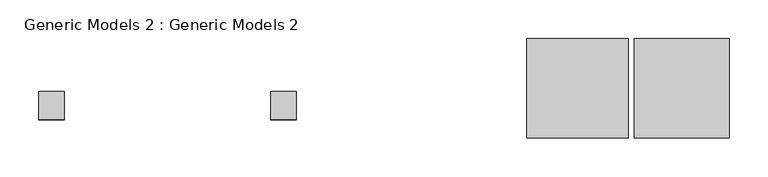
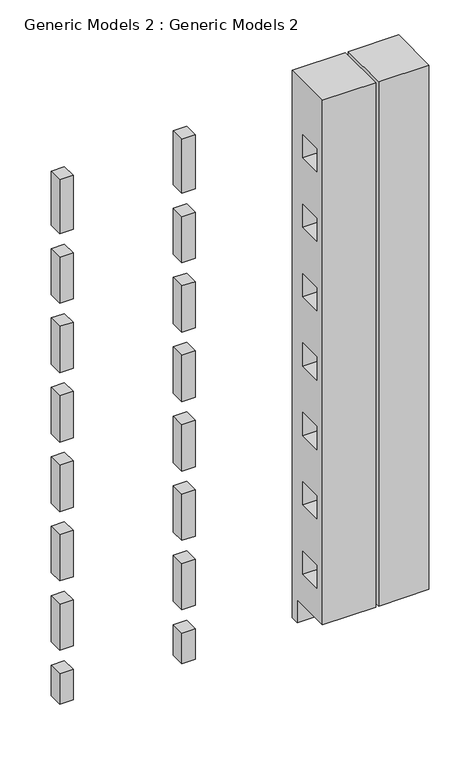
"""IFC4 building model written with IfcOpenShell, lengths in millimetres: proxy geometry, Generic Models 2 : Generic Models 2."""

from ifc_helpers import new_model, si_unit, frame, origin, place, context, project, spatial, polyline, outline, extrude, source, transform, mapped, element, save


def generic_models_2_generic_models_2_e4755291(model_context):
    return source(origin(), model_context, "Body", "SweptSolid", [
        extrude(outline(polyline([(-2976.5029848, -6160.9896754), (-2976.5029848, -6197.2837816), (-3009.36382, -6197.2837816), (-3009.36382, -6160.9896754), (-2976.5029848, -6160.9896754)])), frame((0.0, 0.0, 834.3679056), z_axis=(0.0, 0.0, 1.0), x_axis=(1.0, 0.0, 0.0)), (0.0, 0.0, 1.0), 140.0),
        extrude(outline(polyline([(-2676.5029848, -6160.9896754), (-2676.5029848, -6197.2837816), (-2709.36382, -6197.2837816), (-2709.36382, -6160.9896754), (-2676.5029848, -6160.9896754)])), frame((0.0, 0.0, 834.3679056), z_axis=(0.0, 0.0, 1.0), x_axis=(1.0, 0.0, 0.0)), (0.0, 0.0, 1.0), 140.0),
        extrude(outline(polyline([(-6092.2648653, 974.3679056), (-6092.2648653, -445.6320944), (-6113.8685722, -445.6320944), (-6113.8685722, -385.6320944), (-6220.9896754, -385.6320944), (-6220.9896754, 974.3679056), (-6092.2648653, 974.3679056)]), holes=[polyline([(-6137.2837816, 834.3679056), (-6197.2837816, 834.3679056), (-6197.2837816, 774.3679056), (-6137.2837816, 774.3679056), (-6137.2837816, 834.3679056)]), polyline([(-6137.2837816, 654.3679056), (-6197.2837816, 654.3679056), (-6197.2837816, 594.3679056), (-6137.2837816, 594.3679056), (-6137.2837816, 654.3679056)]), polyline([(-6137.2837816, 474.3679056), (-6197.2837816, 474.3679056), (-6197.2837816, 414.3679056), (-6137.2837816, 414.3679056), (-6137.2837816, 474.3679056)]), polyline([(-6137.2837816, 294.3679056), (-6197.2837816, 294.3679056), (-6197.2837816, 234.3679056), (-6137.2837816, 234.3679056), (-6137.2837816, 294.3679056)]), polyline([(-6137.2837816, 114.3679056), (-6197.2837816, 114.3679056), (-6197.2837816, 54.3679056), (-6137.2837816, 54.3679056), (-6137.2837816, 114.3679056)]), polyline([(-6137.2837816, -65.6320944), (-6197.2837816, -65.6320944), (-6197.2837816, -125.6320944), (-6137.2837816, -125.6320944), (-6137.2837816, -65.6320944)]), polyline([(-6137.2837816, -245.6320944), (-6197.2837816, -245.6320944), (-6197.2837816, -305.6320944), (-6137.2837816, -305.6320944), (-6137.2837816, -245.6320944)])]), frame((-2378.5868425, 0.0, 0.0), z_axis=(1.0, 0.0, 0.0), x_axis=(0.0, 1.0, 0.0)), (0.0, 0.0, 1.0), 130.7324377),
        extrude(outline(polyline([(-6092.2648653, 974.3679056), (-6092.2648653, -445.6320944), (-6113.8685722, -445.6320944), (-6113.8685722, -385.6320944), (-6220.9896754, -385.6320944), (-6220.9896754, 974.3679056), (-6092.2648653, 974.3679056)]), holes=[polyline([(-6137.2837816, 834.3679056), (-6197.2837816, 834.3679056), (-6197.2837816, 774.3679056), (-6137.2837816, 774.3679056), (-6137.2837816, 834.3679056)]), polyline([(-6137.2837816, 654.3679056), (-6197.2837816, 654.3679056), (-6197.2837816, 594.3679056), (-6137.2837816, 594.3679056), (-6137.2837816, 654.3679056)]), polyline([(-6137.2837816, 474.3679056), (-6197.2837816, 474.3679056), (-6197.2837816, 414.3679056), (-6137.2837816, 414.3679056), (-6137.2837816, 474.3679056)]), polyline([(-6137.2837816, 294.3679056), (-6197.2837816, 294.3679056), (-6197.2837816, 234.3679056), (-6137.2837816, 234.3679056), (-6137.2837816, 294.3679056)]), polyline([(-6137.2837816, 114.3679056), (-6197.2837816, 114.3679056), (-6197.2837816, 54.3679056), (-6137.2837816, 54.3679056), (-6137.2837816, 114.3679056)]), polyline([(-6137.2837816, -65.6320944), (-6197.2837816, -65.6320944), (-6197.2837816, -125.6320944), (-6137.2837816, -125.6320944), (-6137.2837816, -65.6320944)]), polyline([(-6137.2837816, -245.6320944), (-6197.2837816, -245.6320944), (-6197.2837816, -305.6320944), (-6137.2837816, -305.6320944), (-6137.2837816, -245.6320944)])]), frame((-2240.2544048, 0.0, 0.0), z_axis=(1.0, 0.0, 0.0), x_axis=(0.0, 1.0, 0.0)), (0.0, 0.0, 1.0), 123.0190663),
        extrude(outline(polyline([(-2976.5029848, -6160.9896754), (-2976.5029848, -6197.2837816), (-3009.36382, -6197.2837816), (-3009.36382, -6160.9896754), (-2976.5029848, -6160.9896754)])), frame((0.0, 0.0, 654.3679056), z_axis=(0.0, 0.0, 1.0), x_axis=(1.0, 0.0, 0.0)), (0.0, 0.0, 1.0), 120.0),
        extrude(outline(polyline([(-2676.5029848, -6160.9896754), (-2676.5029848, -6197.2837816), (-2709.36382, -6197.2837816), (-2709.36382, -6160.9896754), (-2676.5029848, -6160.9896754)])), frame((0.0, 0.0, 654.3679056), z_axis=(0.0, 0.0, 1.0), x_axis=(1.0, 0.0, 0.0)), (0.0, 0.0, 1.0), 120.0),
        extrude(outline(polyline([(-2976.5029848, -6160.9896754), (-2976.5029848, -6197.2837816), (-3009.36382, -6197.2837816), (-3009.36382, -6160.9896754), (-2976.5029848, -6160.9896754)])), frame((0.0, 0.0, 474.3679056), z_axis=(0.0, 0.0, 1.0), x_axis=(1.0, 0.0, 0.0)), (0.0, 0.0, 1.0), 120.0),
        extrude(outline(polyline([(-2676.5029848, -6160.9896754), (-2676.5029848, -6197.2837816), (-2709.36382, -6197.2837816), (-2709.36382, -6160.9896754), (-2676.5029848, -6160.9896754)])), frame((0.0, 0.0, 474.3679056), z_axis=(0.0, 0.0, 1.0), x_axis=(1.0, 0.0, 0.0)), (0.0, 0.0, 1.0), 120.0),
        extrude(outline(polyline([(-2976.5029848, -6160.9896754), (-2976.5029848, -6197.2837816), (-3009.36382, -6197.2837816), (-3009.36382, -6160.9896754), (-2976.5029848, -6160.9896754)])), frame((0.0, 0.0, 294.3679056), z_axis=(0.0, 0.0, 1.0), x_axis=(1.0, 0.0, 0.0)), (0.0, 0.0, 1.0), 120.0),
        extrude(outline(polyline([(-2676.5029848, -6160.9896754), (-2676.5029848, -6197.2837816), (-2709.36382, -6197.2837816), (-2709.36382, -6160.9896754), (-2676.5029848, -6160.9896754)])), frame((0.0, 0.0, 294.3679056), z_axis=(0.0, 0.0, 1.0), x_axis=(1.0, 0.0, 0.0)), (0.0, 0.0, 1.0), 120.0),
        extrude(outline(polyline([(-2976.5029848, -6160.9896754), (-2976.5029848, -6197.2837816), (-3009.36382, -6197.2837816), (-3009.36382, -6160.9896754), (-2976.5029848, -6160.9896754)])), frame((0.0, 0.0, 114.3679056), z_axis=(0.0, 0.0, 1.0), x_axis=(1.0, 0.0, 0.0)), (0.0, 0.0, 1.0), 120.0),
        extrude(outline(polyline([(-2676.5029848, -6160.9896754), (-2676.5029848, -6197.2837816), (-2709.36382, -6197.2837816), (-2709.36382, -6160.9896754), (-2676.5029848, -6160.9896754)])), frame((0.0, 0.0, 114.3679056), z_axis=(0.0, 0.0, 1.0), x_axis=(1.0, 0.0, 0.0)), (0.0, 0.0, 1.0), 120.0),
        extrude(outline(polyline([(-2976.5029848, -6160.9896754), (-2976.5029848, -6197.2837816), (-3009.36382, -6197.2837816), (-3009.36382, -6160.9896754), (-2976.5029848, -6160.9896754)])), frame((0.0, 0.0, -65.6320944), z_axis=(0.0, 0.0, 1.0), x_axis=(1.0, 0.0, 0.0)), (0.0, 0.0, 1.0), 120.0),
        extrude(outline(polyline([(-2676.5029848, -6160.9896754), (-2676.5029848, -6197.2837816), (-2709.36382, -6197.2837816), (-2709.36382, -6160.9896754), (-2676.5029848, -6160.9896754)])), frame((0.0, 0.0, -65.6320944), z_axis=(0.0, 0.0, 1.0), x_axis=(1.0, 0.0, 0.0)), (0.0, 0.0, 1.0), 120.0),
        extrude(outline(polyline([(-2976.5029848, -6160.9896754), (-2976.5029848, -6197.2837816), (-3009.36382, -6197.2837816), (-3009.36382, -6160.9896754), (-2976.5029848, -6160.9896754)])), frame((0.0, 0.0, -245.6320944), z_axis=(0.0, 0.0, 1.0), x_axis=(1.0, 0.0, 0.0)), (0.0, 0.0, 1.0), 120.0),
        extrude(outline(polyline([(-2676.5029848, -6160.9896754), (-2676.5029848, -6197.2837816), (-2709.36382, -6197.2837816), (-2709.36382, -6160.9896754), (-2676.5029848, -6160.9896754)])), frame((0.0, 0.0, -245.6320944), z_axis=(0.0, 0.0, 1.0), x_axis=(1.0, 0.0, 0.0)), (0.0, 0.0, 1.0), 120.0),
        extrude(outline(polyline([(-2976.5029848, -6160.9896754), (-2976.5029848, -6197.2837816), (-3009.36382, -6197.2837816), (-3009.36382, -6160.9896754), (-2976.5029848, -6160.9896754)])), frame((0.0, 0.0, -385.6320944), z_axis=(0.0, 0.0, 1.0), x_axis=(1.0, 0.0, 0.0)), (0.0, 0.0, 1.0), 80.0),
        extrude(outline(polyline([(-2676.5029848, -6160.9896754), (-2676.5029848, -6197.2837816), (-2709.36382, -6197.2837816), (-2709.36382, -6160.9896754), (-2676.5029848, -6160.9896754)])), frame((0.0, 0.0, -385.6320944), z_axis=(0.0, 0.0, 1.0), x_axis=(1.0, 0.0, 0.0)), (0.0, 0.0, 1.0), 80.0),
    ])


if __name__ == "__main__":
    model = new_model("IFC4")
    model_context = context("Model", 3, world=origin())
    ifc_project = project(units=[si_unit("LENGTHUNIT", "METRE", prefix="MILLI")], contexts=[model_context])
    site = spatial("IfcSite", under=ifc_project)
    building = spatial("IfcBuilding", under=site)
    placement = place(None, origin())
    generic_models_2_generic_models_2_shape = generic_models_2_generic_models_2_e4755291(model_context)
    element("IfcBuildingElementProxy", 1, Name="Generic Models 2 : Generic Models 2", ObjectType="Generic Models 2 : Generic Models 2", at=placement, inside=building, context=model_context, shape_type="MappedRepresentation", body=[
        mapped(generic_models_2_generic_models_2_shape, transform((0.0, 0.0, 0.0), x_axis=(1.0, 0.0, 0.0), y_axis=(0.0, 1.0, 0.0), z_axis=(0.0, 0.0, 1.0))),
    ])
    save(model, "model.ifc")
